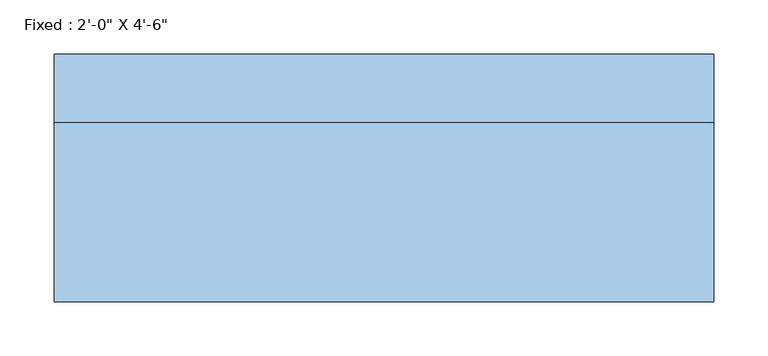
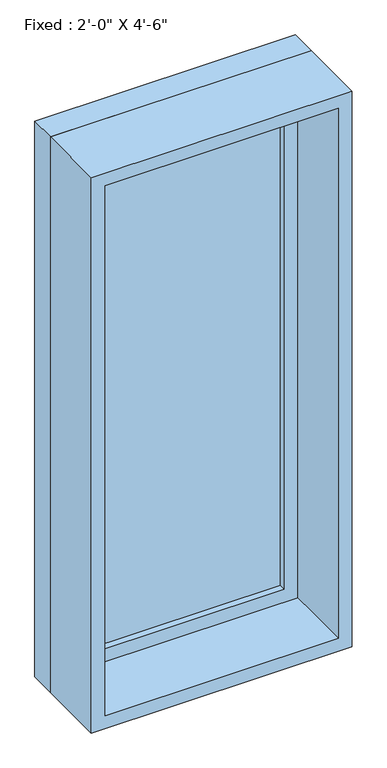
"""IFC4 building model written with IfcOpenShell, lengths in millimetres: window geometry."""

from ifc_helpers import new_model, si_unit, frame, origin, place, context, project, spatial, polyline, outline, extrude, source, transform, mapped, element, save


def window_41ad1500(model_context):
    return source(origin(), model_context, "Body", "SweptSolid", [
        extrude(outline(polyline([(203.2, 66.675), (-279.4, 66.675), (-279.4, 79.375), (203.2, 79.375), (203.2, 66.675)])), frame((0.0, 0.0, 825.5), z_axis=(0.0, 0.0, 1.0), x_axis=(1.0, 0.0, 0.0)), (0.0, 0.0, 1.0), 1244.6),
        extrude(outline(polyline([(2114.55, -323.85), (781.05, -323.85), (781.05, 247.65), (2114.55, 247.65), (2114.55, -323.85)]), holes=[polyline([(2070.1, -279.4), (2070.1, 203.2), (825.5, 203.2), (825.5, -279.4), (2070.1, -279.4)])]), frame((0.0, 50.8, 0.0), z_axis=(0.0, 1.0, 0.0), x_axis=(0.0, 0.0, 1.0)), (0.0, 0.0, 1.0), 44.45),
        extrude(outline(polyline([(2133.6, -342.9), (762.0, -342.9), (762.0, 266.7), (2133.6, 266.7), (2133.6, -342.9)]), holes=[polyline([(2101.85, -311.15), (2101.85, 234.95), (793.75, 234.95), (793.75, -311.15), (2101.85, -311.15)])]), frame((0.0, -114.3, 0.0), z_axis=(0.0, 1.0, 0.0), x_axis=(0.0, 0.0, 1.0)), (0.0, 0.0, 1.0), 165.1),
        extrude(outline(polyline([(2133.6, 266.7), (2133.6, -342.9), (762.0, -342.9), (762.0, 266.7), (2133.6, 266.7)]), holes=[polyline([(2114.55, 247.65), (781.05, 247.65), (781.05, -323.85), (2114.55, -323.85), (2114.55, 247.65)])]), frame((0.0, 50.8, 0.0), z_axis=(0.0, 1.0, 0.0), x_axis=(0.0, 0.0, 1.0)), (0.0, 0.0, 1.0), 63.5),
    ])


if __name__ == "__main__":
    model = new_model("IFC4")
    model_context = context("Model", 3, world=origin())
    ifc_project = project(units=[si_unit("LENGTHUNIT", "METRE", prefix="MILLI")], contexts=[model_context])
    site = spatial("IfcSite", under=ifc_project)
    building = spatial("IfcBuilding", under=site)
    placement = place(None, origin())
    window_shape = window_41ad1500(model_context)
    element("IfcWindow", 1, ObjectType="Fixed : 2'-0\" X 4'-6\"", at=placement, inside=building, context=model_context, shape_type="MappedRepresentation", body=[
        mapped(window_shape, transform((0.0, 0.0, 0.0), x_axis=(1.0, 0.0, 0.0), y_axis=(0.0, 1.0, 0.0), z_axis=(0.0, 0.0, 1.0))),
    ])
    save(model, "model.ifc")

# Revit data of these elements
# Type "Fixed : 2'-0\" X 4'-6\""
#   Type Mark = "22"
#   Construction Type Id = "GSP4R"
#   Assembly Code = "B2020100"
#   Analytic Construction = "1/8 in Pilkington single glazing"
#   Visual Light Transmittance = 0.9
#   Solar Heat Gain Coefficient = 0.78
#   Heat Transfer Coefficient (U) = 0.6496 BTU/(h·ft²·°F)
#   Height = 4' - 6"
#   Default Sill Height = 2' - 6"
#   Width = 2' - 0"
#   Window Inset = 0' - 0 3/4"
#   Define Thermal Properties by = 1
#   Glass Pane Material = Glass
#   Sash Material = Sash
#   Wall Closure = (empty or 0)
# Element 1 (IfcWindow, "Fixed : 2'-0\" X 4'-6\"")
#   Materials on its faces: "Sash", "Glass"
# Materials
#   "Glass": class "Glass", colour RGB 0 128 192, transparency 0.75, Description = "Soda Lime Glass", Cost = 0
#   "Sash": class "Wood", colour RGB 224 178 126, transparency 0, Cost = 0
